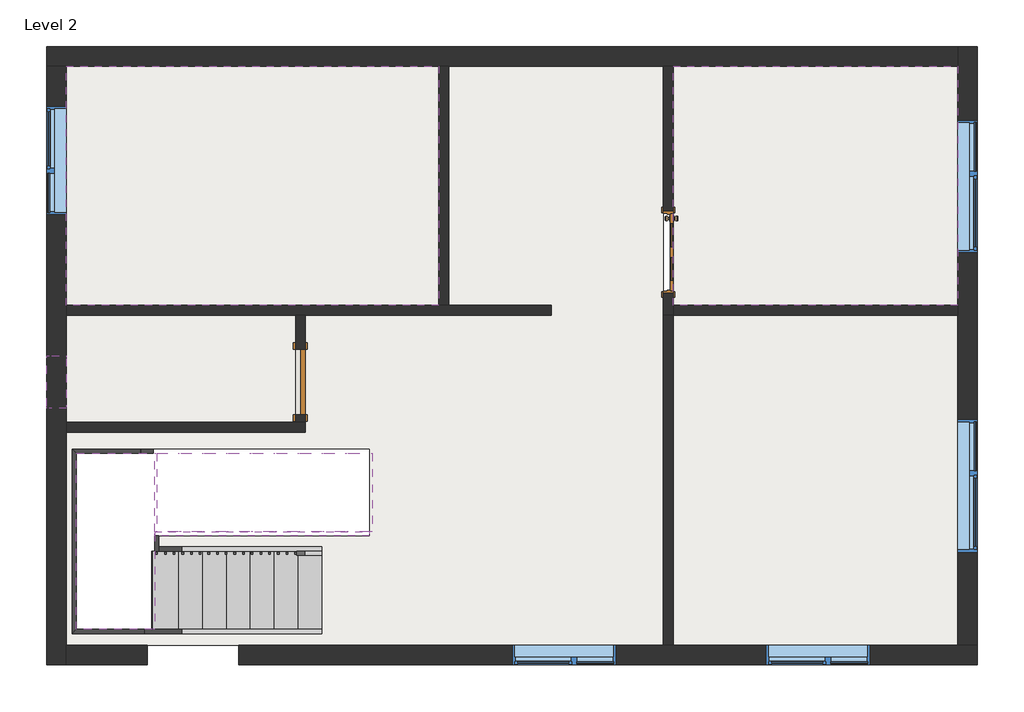
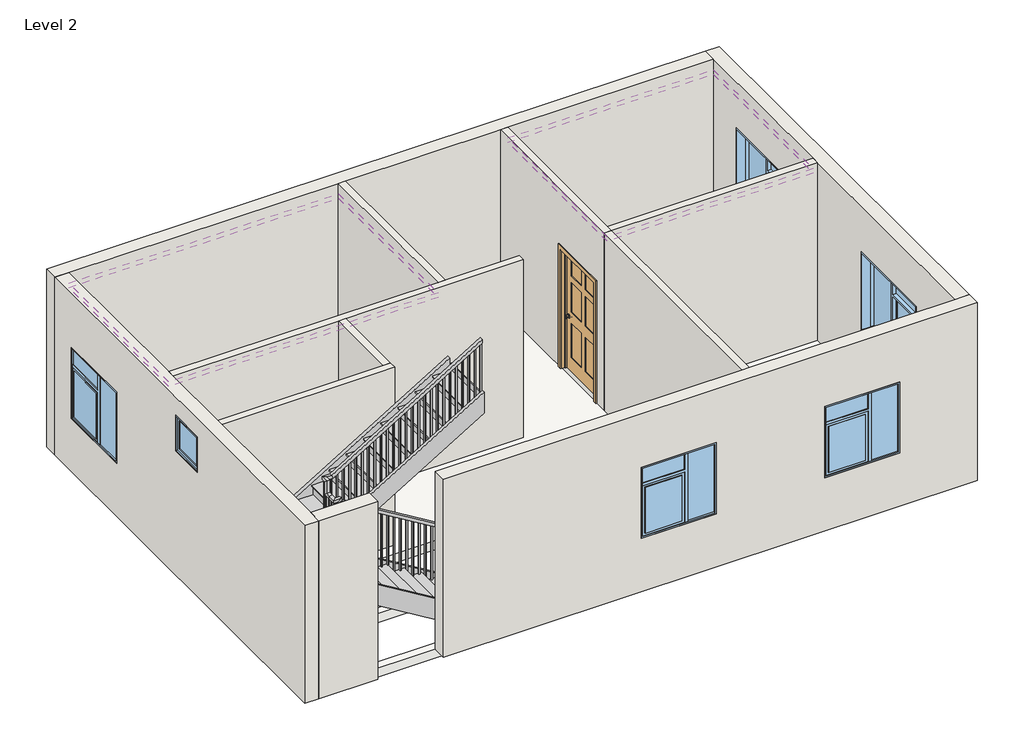
# One storey: 11 walls, 8 members, 6 windows, 4 coverings, 2 doors, 2 slabs, 2 stair flights, 1 railing.
# Revit data of these elements (continued)
# Elements 7, 8, 9, 10, 11, 12, 13, 14 (IfcMember, "Stringer - 2\" Width")
#   Phase Created = New Construction
# Element 15 (IfcRailing, "Handrail - Rectangular")
#   Phase Created = New Construction
# Element 16 (IfcSlab, "FLOORING 6\"")
#   Height Offset From Level = 0' - 0"
#   Phase Created = New Construction
#   Materials on its faces: "FLOORING 1'"
# Element 17 (IfcSlab, "Non-Monolithic Landing")
#   Phase Created = New Construction
# Elements 18, 19 (IfcStairFlight, "2\" Tread 1\" Nosing 1/4\" Riser")
#   Phase Created = New Construction
# Elements 20, 21, 22, 23 (IfcWall, "OUTER Wall 9\"")
#   Top Offset = 0' - 0"
#   Base Offset = 0' - 0"
#   wall height = 10' - 0"
#   Phase Created = New Construction
#   Base Constraint = Level 2
#   Top Constraint = Level 4
#   Materials on its faces: "outer wall"
# Elements 24, 25, 26, 27, 28, 29, 30 (IfcWall, "inner wall 4.5\"")
#   Top Offset = 0' - 0"
#   Base Offset = 0' - 0"
#   wall height = 10' - 0"
#   Phase Created = New Construction
#   Base Constraint = Level 2
#   Top Constraint = Level 4
#   Materials on its faces: "outer wall"
# Element 31 (IfcWindow, "Fixed : 24\" x 24\"")
#   Mark = "7"
#   Phase Created = New Construction
#   Materials on its faces: "Sash", "Glass"
# Element 32 (IfcWindow, "Window-Casement-Double-Sidelight : 50\" x 48\"")
#   Mark = "10"
#   Window Inset = 0' - 0 5/8"
#   Frame Gap 3 = 0' - 1 83/128"
#   Frame Gap 2 = 0' - 0 5/8"
#   Phase Created = New Construction
#   Materials on its faces: "Metal - Aluminum", "Glass"
# Element 33 (IfcWindow, "Window-Casement-Double-Sidelight : 61\" x 53\"")
#   Mark = "8"
#   Window Inset = 0' - 0 5/8"
#   Frame Gap 3 = 0' - 1 83/128"
#   Frame Gap 2 = 0' - 0 5/8"
#   Phase Created = New Construction
#   Materials on its faces: "Metal - Aluminum", "Glass"
# Element 34 (IfcWindow, "Window-Casement-Double-Sidelight : 61\" x 53\"")
#   Mark = "9"
#   Window Inset = 0' - 0 5/8"
#   Frame Gap 3 = 0' - 1 83/128"
#   Frame Gap 2 = 0' - 0 5/8"
#   Phase Created = New Construction
#   Materials on its faces: "Metal - Aluminum", "Glass"
# Element 35 (IfcWindow, "Window-Casement-Double-Sidelight : WINDOWS 4' X 4' 2")
#   Mark = "11"
#   Window Inset = 0' - 0 5/8"
#   Frame Gap 3 = 0' - 1 83/128"
#   Frame Gap 2 = 0' - 0 5/8"
#   Phase Created = New Construction
#   Materials on its faces: "BLACK MATERIAL", "Glass"
# Element 36 (IfcWindow, "Window-Casement-Double-Sidelight : WINDOWS 4' X 4' 2")
#   Mark = "12"
#   Window Inset = 0' - 0 5/8"
#   Frame Gap 3 = 0' - 1 83/128"
#   Frame Gap 2 = 0' - 0 5/8"
#   Phase Created = New Construction
#   Materials on its faces: "BLACK MATERIAL", "Glass"
# Materials
#   "Metal Stud Layer": class "Metal", colour RGB 199 199 199, transparency 0, Description = "Light gauge steel framing, thermal air layer", Cost = 0
#   "Laminate, Ivory, Matte": class "Plastic", colour RGB 247 247 239, transparency 0, Description = "Plastic Laminate - Ivory, Matte", Cost = 0
#   "Cherry": class "Wood", colour RGB 226 177 128, transparency 0, Description = "Prunus Serotina", Cost = 0
#   "Aluminum": class "Metal", colour RGB 247 247 247, transparency 0, Description = "Aluminum 6061", Cost = 0
#   "Door - Panel": class "Wood", colour RGB 210 159 95, transparency 0, Cost = 0
#   "Door - Frame": colour RGB 118 70 51, transparency 0, Cost = 0
#   "FLOORING 1'": class "Generic", colour RGB 120 120 120, transparency 0, Cost = 0
#   "outer wall": class "Generic", colour RGB 120 120 120, transparency 0, Cost = 0
#   "Glass": class "Glass", colour RGB 0 128 192, transparency 0.75, Description = "Soda Lime Glass", Cost = 0
#   "Sash": class "Wood", colour RGB 224 178 126, transparency 0, Cost = 0
#   "Metal - Aluminum": class "Metal", colour RGB 247 247 247, transparency 0
#   "BLACK MATERIAL": class "Generic", colour RGB 120 120 120, transparency 0, Cost = 0
